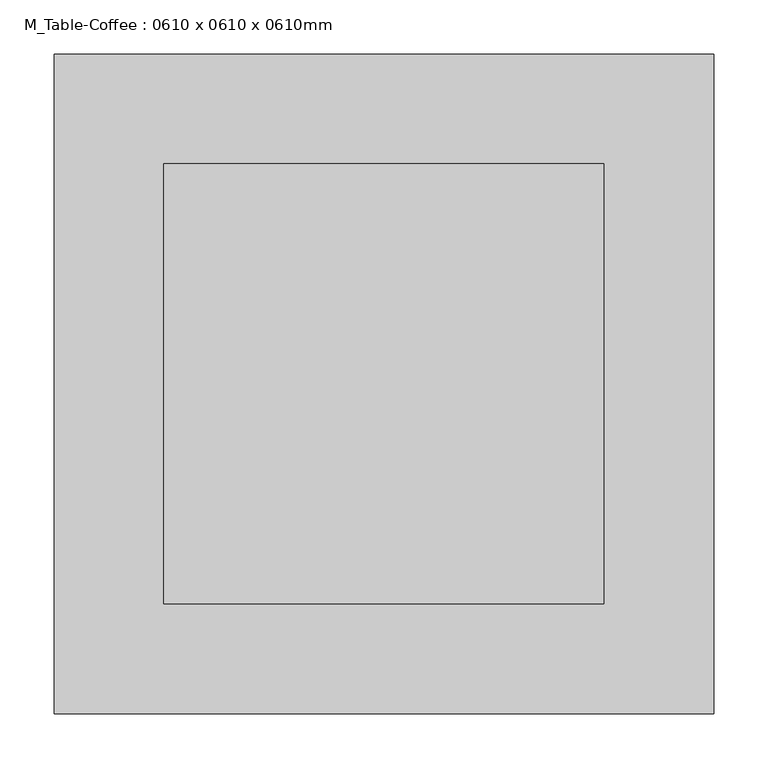
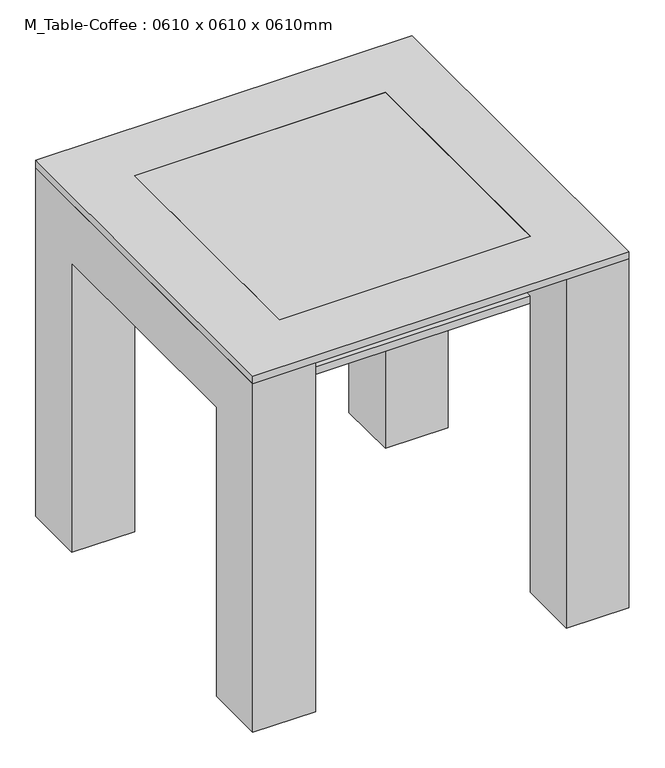
"""IFC4 building model written with IfcOpenShell, lengths in millimetres: furniture geometry, M_Table-Coffee : 0610 x 0610 x 0610mm."""

from ifc_helpers import new_model, si_unit, frame, origin, place, context, project, spatial, polyline, outline, extrude, source, transform, mapped, element, save


def m_table_coffee_0610_x_0610_x_0610mm_038d1558(model_context):
    return source(origin(), model_context, "Body", "SweptSolid", [
        extrude(outline(polyline([(323.2657667, 400.2110778), (323.2657667, -209.7889222), (-286.7342333, -209.7889222), (-286.7342333, 400.2110778), (323.2657667, 400.2110778)]), holes=[polyline([(221.6657667, 298.6110778), (-185.1342333, 298.6110778), (-185.1342333, -108.1889222), (221.6657667, -108.1889222), (221.6657667, 298.6110778)])]), frame((0.0, 0.0, 597.3), z_axis=(0.0, 0.0, 1.0), x_axis=(1.0, 0.0, 0.0)), (0.0, 0.0, 1.0), 12.7),
        extrude(outline(polyline([(221.6657667, 298.6110778), (221.6657667, -108.1889222), (-185.1342333, -108.1889222), (-185.1342333, 298.6110778), (221.6657667, 298.6110778)])), frame((0.0, 0.0, 597.3), z_axis=(0.0, 0.0, 1.0), x_axis=(1.0, 0.0, 0.0)), (0.0, 0.0, 1.0), 12.7),
        extrude(outline(polyline([(400.2110778, 597.3), (400.2110778, 0.0), (298.6110778, 0.0), (298.6110778, 495.7), (-108.1889222, 495.7), (-108.1889222, 0.0), (-209.7889222, 0.0), (-209.7889222, 597.3), (400.2110778, 597.3)])), frame((-286.7342333, 0.0, 0.0), z_axis=(1.0, 0.0, 0.0), x_axis=(0.0, 1.0, 0.0)), (0.0, 0.0, 1.0), 101.6),
        extrude(outline(polyline([(400.2110778, 0.0), (298.6110778, 0.0), (298.6110778, 495.7), (-108.1889222, 495.7), (-108.1889222, 0.0), (-209.7889222, 0.0), (-209.7889222, 597.3), (400.2110778, 597.3), (400.2110778, 0.0)])), frame((221.6657667, 0.0, 0.0), z_axis=(1.0, 0.0, 0.0), x_axis=(0.0, 1.0, 0.0)), (0.0, 0.0, 1.0), 101.6),
        extrude(outline(polyline([(221.6657667, 298.6110778), (221.6657667, -108.1889222), (-185.1342333, -108.1889222), (-185.1342333, 298.6110778), (221.6657667, 298.6110778)])), frame((0.0, 0.0, 495.7), z_axis=(0.0, 0.0, 1.0), x_axis=(1.0, 0.0, 0.0)), (0.0, 0.0, 1.0), 12.7),
    ])


if __name__ == "__main__":
    model = new_model("IFC4")
    model_context = context("Model", 3, world=origin())
    ifc_project = project(units=[si_unit("LENGTHUNIT", "METRE", prefix="MILLI")], contexts=[model_context])
    site = spatial("IfcSite", under=ifc_project)
    building = spatial("IfcBuilding", under=site)
    placement = place(None, origin())
    m_table_coffee_0610_x_0610_x_0610mm_shape = m_table_coffee_0610_x_0610_x_0610mm_038d1558(model_context)
    element("IfcFurniture", 1, ObjectType="M_Table-Coffee : 0610 x 0610 x 0610mm", at=placement, inside=building, context=model_context, shape_type="MappedRepresentation", body=[
        mapped(m_table_coffee_0610_x_0610_x_0610mm_shape, transform((0.0, 0.0, 0.0), x_axis=(1.0, 0.0, 0.0), y_axis=(0.0, 1.0, 0.0), z_axis=(0.0, 0.0, 1.0))),
    ])
    save(model, "model.ifc")

# Revit data of these elements
# Type "M_Table-Coffee : 0610 x 0610 x 0610mm"
#   Height = 610 mm
#   Length = 610 mm
#   Width = 610 mm
#   Top Material = Steel, Chrome Plated
#   Frame Material = Wood - Teak
#   Default Elevation = 0
# Element 1 (IfcFurniture, "M_Table-Coffee : 0610 x 0610 x 0610mm")
#   Materials on its faces: "Wood - Teak", "Steel, Chrome Plated", "Glass - Clear, Grey"
# Materials
#   "Steel, Chrome Plated": class "Metal", colour RGB 17 17 17, transparency 0, Description = "Chromiuim plated steel", Cost = 0
#   "Wood - Teak": class "Wood", colour RGB 145 112 90, transparency 0
#   "Glass - Clear, Grey": class "Glass", colour RGB 252 255 255, transparency 0.64
